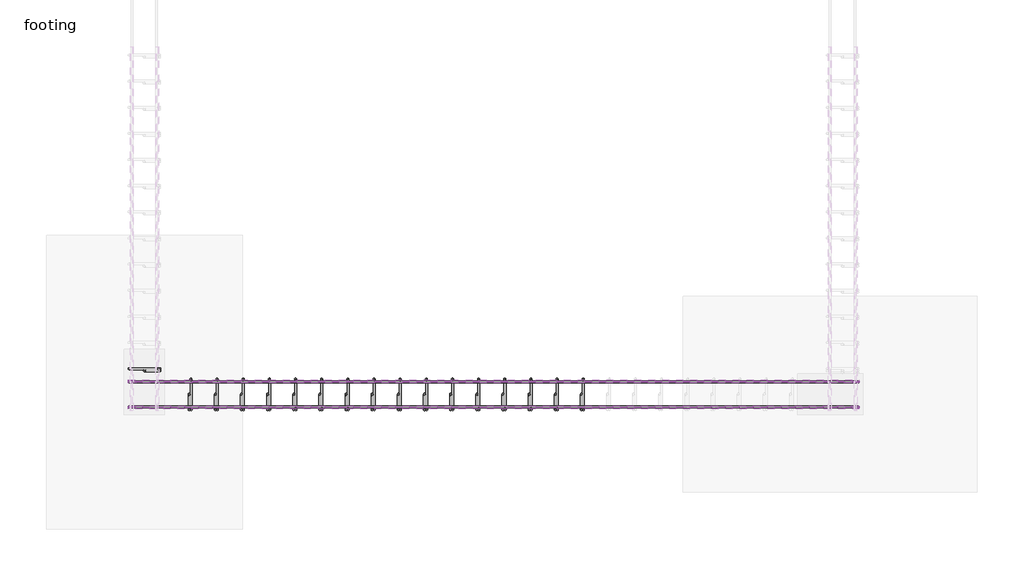
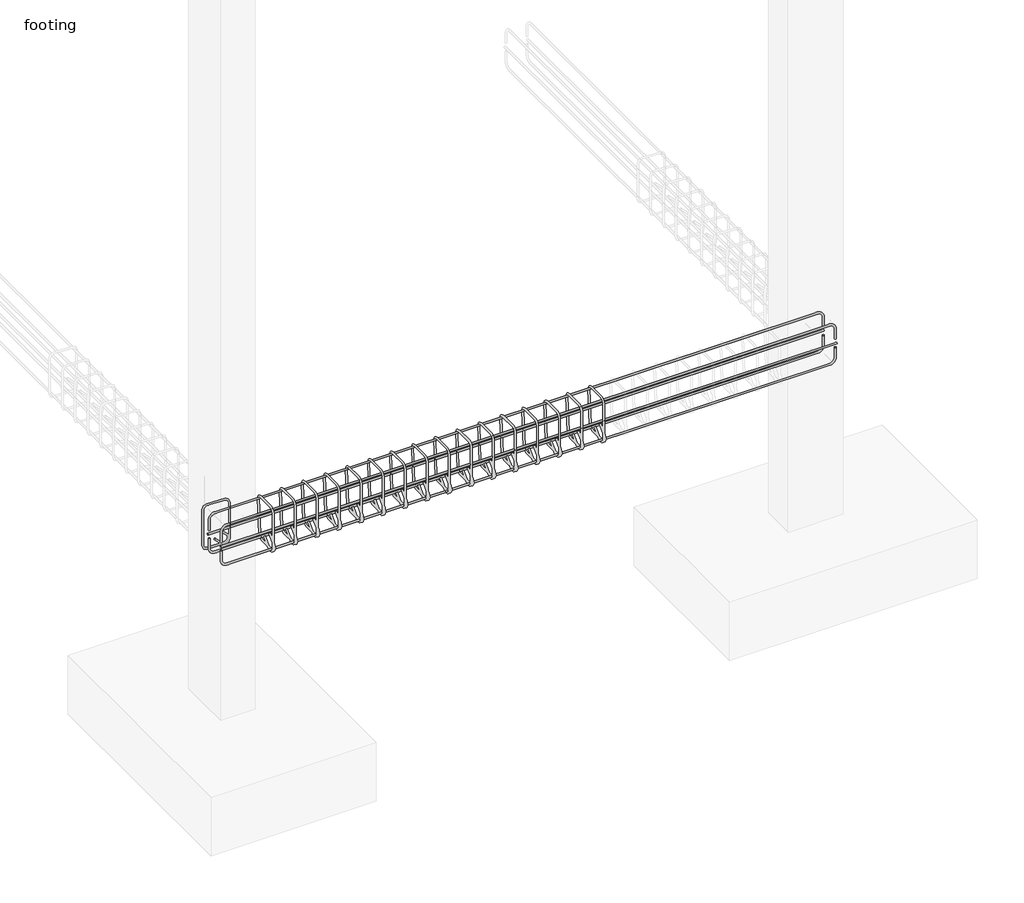
# One storey, part 2 of 21: 23 reinforcing bars.
"""IFC4 building model written with IfcOpenShell, lengths in millimetres."""

from ifc_helpers import new_model, si_unit, point, frame, origin, place, context, project, spatial, polyline, circle_curve, trimmed, segment, composite_curve, element, save
from ifc_brep_helpers import swept_disk

model = new_model("IFC4")

# Units and contexts
model_context = context("Model", 3, world=origin())
ifc_project = project(units=[si_unit("LENGTHUNIT", "METRE", prefix="MILLI")], contexts=[model_context])

# Site, building, storey
site = spatial("IfcSite", under=ifc_project)
building = spatial("IfcBuilding", under=site)
storey = spatial("IfcBuildingStorey", under=building, Name="footing", Elevation=-1524.0)

# Reinforcing bars
placement = place(None, origin())
element("IfcReinforcingBar", 1, at=placement, inside=storey, context=model_context, shape_type="SolidModel", body=[
    swept_disk(composite_curve([segment(polyline([(-11932.2883428, -282.6612868, -310.8825168), (-11932.2883428, -337.5262853, -365.7475153)]), True, "CONTINUOUS"), segment(trimmed(circle_curve(frame((-11932.2883428, -359.9769256, -343.296875), z_axis=(-1.0, 0.0, 0.0), x_axis=(0.0, 22.450640300000032, -22.450640299999975)), 31.75), [point((-11932.2883428, -337.5262853, -365.7475153))], [point((-11932.2883428, -391.7269256, -343.296875))], True, "CARTESIAN"), True, "CONTINUOUS"), segment(polyline([(-11932.2883428, -391.7269256, -343.296875), (-11932.2883428, -391.7269256, -63.103125)]), True, "CONTINUOUS"), segment(trimmed(circle_curve(frame((-11932.2883428, -359.9769256, -63.103125), z_axis=(-1.0, 0.0, 0.0), x_axis=(0.0, -31.75, 0.0)), 31.75), [point((-11932.2883428, -391.7269256, -63.103125))], [point((-11932.2883428, -359.9769256, -31.353125))], True, "CARTESIAN"), True, "CONTINUOUS"), segment(polyline([(-11932.2883428, -359.9769256, -31.353125), (-11932.2883428, -232.1831756, -31.353125)]), True, "CONTINUOUS"), segment(trimmed(circle_curve(frame((-11931.1159328, -232.1831756, -63.0814712), z_axis=(-0.9993179916193466, 0.0, -0.03692629992126919), x_axis=(-1.1724100000010367, 0.0, 31.728346200000004)), 31.75), [point((-11932.2883428, -232.1831756, -31.353125))], [point((-11931.1159328, -200.4331756, -63.0814712))], True, "CARTESIAN"), True, "CONTINUOUS"), segment(polyline([(-11931.1159328, -200.4331756, -63.0814712), (-11920.7607528, -200.4331756, -343.3185288)]), True, "CONTINUOUS"), segment(trimmed(circle_curve(frame((-11920.7607528, -232.1831756, -343.3185288), z_axis=(-0.9993179916193466, 0.0, -0.03692629992126919), x_axis=(0.0, 31.75, 0.0)), 31.75), [point((-11920.7607528, -200.4331756, -343.3185288))], [point((-11919.5883428, -232.1831756, -375.046875))], True, "CARTESIAN"), True, "CONTINUOUS"), segment(polyline([(-11919.5883428, -232.1831756, -375.046875), (-11919.5883428, -359.9769256, -375.046875)]), True, "CONTINUOUS"), segment(trimmed(circle_curve(frame((-11919.5883428, -359.9769256, -343.296875), z_axis=(-1.0, 0.0, 0.0), x_axis=(0.0, 0.0, -31.75)), 31.75), [point((-11919.5883428, -359.9769256, -375.046875))], [point((-11919.5883428, -382.4275659, -320.8462347))], True, "CARTESIAN"), True, "CONTINUOUS"), segment(polyline([(-11919.5883428, -382.4275659, -320.8462347), (-11919.5883428, -327.5625674, -265.9812362)]), True, "CONTINUOUS")], self_intersect=False), 6.35),
])
element("IfcReinforcingBar", 2, at=placement, inside=storey, context=model_context, shape_type="SolidModel", body=[
    swept_disk(composite_curve([segment(polyline([(-11769.5883428, -282.6612868, -310.8825168), (-11769.5883428, -337.5262853, -365.7475153)]), True, "CONTINUOUS"), segment(trimmed(circle_curve(frame((-11769.5883428, -359.9769256, -343.296875), z_axis=(-1.0, 0.0, 0.0), x_axis=(0.0, 22.450640300000032, -22.450640299999975)), 31.75), [point((-11769.5883428, -337.5262853, -365.7475153))], [point((-11769.5883428, -391.7269256, -343.296875))], True, "CARTESIAN"), True, "CONTINUOUS"), segment(polyline([(-11769.5883428, -391.7269256, -343.296875), (-11769.5883428, -391.7269256, -63.103125)]), True, "CONTINUOUS"), segment(trimmed(circle_curve(frame((-11769.5883428, -359.9769256, -63.103125), z_axis=(-1.0, 0.0, 0.0), x_axis=(0.0, -31.75, 0.0)), 31.75), [point((-11769.5883428, -391.7269256, -63.103125))], [point((-11769.5883428, -359.9769256, -31.353125))], True, "CARTESIAN"), True, "CONTINUOUS"), segment(polyline([(-11769.5883428, -359.9769256, -31.353125), (-11769.5883428, -232.1831756, -31.353125)]), True, "CONTINUOUS"), segment(trimmed(circle_curve(frame((-11768.4159328, -232.1831756, -63.0814712), z_axis=(-0.9993179916193466, 0.0, -0.03692629992126919), x_axis=(-1.1724099999992177, 0.0, 31.728346200000004)), 31.75), [point((-11769.5883428, -232.1831756, -31.353125))], [point((-11768.4159328, -200.4331756, -63.0814712))], True, "CARTESIAN"), True, "CONTINUOUS"), segment(polyline([(-11768.4159328, -200.4331756, -63.0814712), (-11758.0607528, -200.4331756, -343.3185288)]), True, "CONTINUOUS"), segment(trimmed(circle_curve(frame((-11758.0607528, -232.1831756, -343.3185288), z_axis=(-0.9993179916193466, 0.0, -0.03692629992126919), x_axis=(0.0, 31.75, 0.0)), 31.75), [point((-11758.0607528, -200.4331756, -343.3185288))], [point((-11756.8883428, -232.1831756, -375.046875))], True, "CARTESIAN"), True, "CONTINUOUS"), segment(polyline([(-11756.8883428, -232.1831756, -375.046875), (-11756.8883428, -359.9769256, -375.046875)]), True, "CONTINUOUS"), segment(trimmed(circle_curve(frame((-11756.8883428, -359.9769256, -343.296875), z_axis=(-1.0, 0.0, 0.0), x_axis=(0.0, 0.0, -31.75)), 31.75), [point((-11756.8883428, -359.9769256, -375.046875))], [point((-11756.8883428, -382.4275659, -320.8462347))], True, "CARTESIAN"), True, "CONTINUOUS"), segment(polyline([(-11756.8883428, -382.4275659, -320.8462347), (-11756.8883428, -327.5625674, -265.9812362)]), True, "CONTINUOUS")], self_intersect=False), 6.35),
])
element("IfcReinforcingBar", 3, at=placement, inside=storey, context=model_context, shape_type="SolidModel", body=[
    swept_disk(composite_curve([segment(polyline([(-11606.8883428, -282.6612868, -310.8825168), (-11606.8883428, -337.5262853, -365.7475153)]), True, "CONTINUOUS"), segment(trimmed(circle_curve(frame((-11606.8883428, -359.9769256, -343.296875), z_axis=(-1.0, 0.0, 0.0), x_axis=(0.0, 22.450640300000032, -22.450640299999975)), 31.75), [point((-11606.8883428, -337.5262853, -365.7475153))], [point((-11606.8883428, -391.7269256, -343.296875))], True, "CARTESIAN"), True, "CONTINUOUS"), segment(polyline([(-11606.8883428, -391.7269256, -343.296875), (-11606.8883428, -391.7269256, -63.103125)]), True, "CONTINUOUS"), segment(trimmed(circle_curve(frame((-11606.8883428, -359.9769256, -63.103125), z_axis=(-1.0, 0.0, 0.0), x_axis=(0.0, -31.75, 0.0)), 31.75), [point((-11606.8883428, -391.7269256, -63.103125))], [point((-11606.8883428, -359.9769256, -31.353125))], True, "CARTESIAN"), True, "CONTINUOUS"), segment(polyline([(-11606.8883428, -359.9769256, -31.353125), (-11606.8883428, -232.1831756, -31.353125)]), True, "CONTINUOUS"), segment(trimmed(circle_curve(frame((-11605.7159328, -232.1831756, -63.0814712), z_axis=(-0.9993179916193466, 0.0, -0.03692629992126919), x_axis=(-1.1724100000010367, 0.0, 31.728346200000004)), 31.75), [point((-11606.8883428, -232.1831756, -31.353125))], [point((-11605.7159328, -200.4331756, -63.0814712))], True, "CARTESIAN"), True, "CONTINUOUS"), segment(polyline([(-11605.7159328, -200.4331756, -63.0814712), (-11595.3607528, -200.4331756, -343.3185288)]), True, "CONTINUOUS"), segment(trimmed(circle_curve(frame((-11595.3607528, -232.1831756, -343.3185288), z_axis=(-0.9993179916193466, 0.0, -0.03692629992126919), x_axis=(0.0, 31.75, 0.0)), 31.75), [point((-11595.3607528, -200.4331756, -343.3185288))], [point((-11594.1883428, -232.1831756, -375.046875))], True, "CARTESIAN"), True, "CONTINUOUS"), segment(polyline([(-11594.1883428, -232.1831756, -375.046875), (-11594.1883428, -359.9769256, -375.046875)]), True, "CONTINUOUS"), segment(trimmed(circle_curve(frame((-11594.1883428, -359.9769256, -343.296875), z_axis=(-1.0, 0.0, 0.0), x_axis=(0.0, 0.0, -31.75)), 31.75), [point((-11594.1883428, -359.9769256, -375.046875))], [point((-11594.1883428, -382.4275659, -320.8462347))], True, "CARTESIAN"), True, "CONTINUOUS"), segment(polyline([(-11594.1883428, -382.4275659, -320.8462347), (-11594.1883428, -327.5625674, -265.9812362)]), True, "CONTINUOUS")], self_intersect=False), 6.35),
])
element("IfcReinforcingBar", 4, at=placement, inside=storey, context=model_context, shape_type="SolidModel", body=[
    swept_disk(composite_curve([segment(polyline([(-11444.1883428, -282.6612868, -310.8825168), (-11444.1883428, -337.5262853, -365.7475153)]), True, "CONTINUOUS"), segment(trimmed(circle_curve(frame((-11444.1883428, -359.9769256, -343.296875), z_axis=(-1.0, 0.0, 0.0), x_axis=(0.0, 22.450640300000032, -22.450640299999975)), 31.75), [point((-11444.1883428, -337.5262853, -365.7475153))], [point((-11444.1883428, -391.7269256, -343.296875))], True, "CARTESIAN"), True, "CONTINUOUS"), segment(polyline([(-11444.1883428, -391.7269256, -343.296875), (-11444.1883428, -391.7269256, -63.103125)]), True, "CONTINUOUS"), segment(trimmed(circle_curve(frame((-11444.1883428, -359.9769256, -63.103125), z_axis=(-1.0, 0.0, 0.0), x_axis=(0.0, -31.75, 0.0)), 31.75), [point((-11444.1883428, -391.7269256, -63.103125))], [point((-11444.1883428, -359.9769256, -31.353125))], True, "CARTESIAN"), True, "CONTINUOUS"), segment(polyline([(-11444.1883428, -359.9769256, -31.353125), (-11444.1883428, -232.1831756, -31.353125)]), True, "CONTINUOUS"), segment(trimmed(circle_curve(frame((-11443.0159328, -232.1831756, -63.0814712), z_axis=(-0.9993179916193466, 0.0, -0.03692629992126919), x_axis=(-1.1724099999992177, 0.0, 31.728346200000004)), 31.75), [point((-11444.1883428, -232.1831756, -31.353125))], [point((-11443.0159328, -200.4331756, -63.0814712))], True, "CARTESIAN"), True, "CONTINUOUS"), segment(polyline([(-11443.0159328, -200.4331756, -63.0814712), (-11432.6607528, -200.4331756, -343.3185288)]), True, "CONTINUOUS"), segment(trimmed(circle_curve(frame((-11432.6607528, -232.1831756, -343.3185288), z_axis=(-0.9993179916193466, 0.0, -0.03692629992126919), x_axis=(0.0, 31.75, 0.0)), 31.75), [point((-11432.6607528, -200.4331756, -343.3185288))], [point((-11431.4883428, -232.1831756, -375.046875))], True, "CARTESIAN"), True, "CONTINUOUS"), segment(polyline([(-11431.4883428, -232.1831756, -375.046875), (-11431.4883428, -359.9769256, -375.046875)]), True, "CONTINUOUS"), segment(trimmed(circle_curve(frame((-11431.4883428, -359.9769256, -343.296875), z_axis=(-1.0, 0.0, 0.0), x_axis=(0.0, 0.0, -31.75)), 31.75), [point((-11431.4883428, -359.9769256, -375.046875))], [point((-11431.4883428, -382.4275659, -320.8462347))], True, "CARTESIAN"), True, "CONTINUOUS"), segment(polyline([(-11431.4883428, -382.4275659, -320.8462347), (-11431.4883428, -327.5625674, -265.9812362)]), True, "CONTINUOUS")], self_intersect=False), 6.35),
])
element("IfcReinforcingBar", 5, at=placement, inside=storey, context=model_context, shape_type="SolidModel", body=[
    swept_disk(composite_curve([segment(polyline([(-11281.4883428, -282.6612868, -310.8825168), (-11281.4883428, -337.5262853, -365.7475153)]), True, "CONTINUOUS"), segment(trimmed(circle_curve(frame((-11281.4883428, -359.9769256, -343.296875), z_axis=(-1.0, 0.0, 0.0), x_axis=(0.0, 22.450640300000032, -22.450640299999975)), 31.75), [point((-11281.4883428, -337.5262853, -365.7475153))], [point((-11281.4883428, -391.7269256, -343.296875))], True, "CARTESIAN"), True, "CONTINUOUS"), segment(polyline([(-11281.4883428, -391.7269256, -343.296875), (-11281.4883428, -391.7269256, -63.103125)]), True, "CONTINUOUS"), segment(trimmed(circle_curve(frame((-11281.4883428, -359.9769256, -63.103125), z_axis=(-1.0, 0.0, 0.0), x_axis=(0.0, -31.75, 0.0)), 31.75), [point((-11281.4883428, -391.7269256, -63.103125))], [point((-11281.4883428, -359.9769256, -31.353125))], True, "CARTESIAN"), True, "CONTINUOUS"), segment(polyline([(-11281.4883428, -359.9769256, -31.353125), (-11281.4883428, -232.1831756, -31.353125)]), True, "CONTINUOUS"), segment(trimmed(circle_curve(frame((-11280.3159328, -232.1831756, -63.0814712), z_axis=(-0.9993179916193466, 0.0, -0.03692629992126919), x_axis=(-1.1724099999992177, 0.0, 31.728346200000004)), 31.75), [point((-11281.4883428, -232.1831756, -31.353125))], [point((-11280.3159328, -200.4331756, -63.0814712))], True, "CARTESIAN"), True, "CONTINUOUS"), segment(polyline([(-11280.3159328, -200.4331756, -63.0814712), (-11269.9607528, -200.4331756, -343.3185288)]), True, "CONTINUOUS"), segment(trimmed(circle_curve(frame((-11269.9607528, -232.1831756, -343.3185288), z_axis=(-0.9993179916193466, 0.0, -0.03692629992126919), x_axis=(0.0, 31.75, 0.0)), 31.75), [point((-11269.9607528, -200.4331756, -343.3185288))], [point((-11268.7883428, -232.1831756, -375.046875))], True, "CARTESIAN"), True, "CONTINUOUS"), segment(polyline([(-11268.7883428, -232.1831756, -375.046875), (-11268.7883428, -359.9769256, -375.046875)]), True, "CONTINUOUS"), segment(trimmed(circle_curve(frame((-11268.7883428, -359.9769256, -343.296875), z_axis=(-1.0, 0.0, 0.0), x_axis=(0.0, 0.0, -31.75)), 31.75), [point((-11268.7883428, -359.9769256, -375.046875))], [point((-11268.7883428, -382.4275659, -320.8462347))], True, "CARTESIAN"), True, "CONTINUOUS"), segment(polyline([(-11268.7883428, -382.4275659, -320.8462347), (-11268.7883428, -327.5625674, -265.9812362)]), True, "CONTINUOUS")], self_intersect=False), 6.35),
])
element("IfcReinforcingBar", 6, at=placement, inside=storey, context=model_context, shape_type="SolidModel", body=[
    swept_disk(composite_curve([segment(polyline([(-11118.7883428, -282.6612868, -310.8825168), (-11118.7883428, -337.5262853, -365.7475153)]), True, "CONTINUOUS"), segment(trimmed(circle_curve(frame((-11118.7883428, -359.9769256, -343.296875), z_axis=(-1.0, 0.0, 0.0), x_axis=(0.0, 22.450640300000032, -22.450640299999975)), 31.75), [point((-11118.7883428, -337.5262853, -365.7475153))], [point((-11118.7883428, -391.7269256, -343.296875))], True, "CARTESIAN"), True, "CONTINUOUS"), segment(polyline([(-11118.7883428, -391.7269256, -343.296875), (-11118.7883428, -391.7269256, -63.103125)]), True, "CONTINUOUS"), segment(trimmed(circle_curve(frame((-11118.7883428, -359.9769256, -63.103125), z_axis=(-1.0, 0.0, 0.0), x_axis=(0.0, -31.75, 0.0)), 31.75), [point((-11118.7883428, -391.7269256, -63.103125))], [point((-11118.7883428, -359.9769256, -31.353125))], True, "CARTESIAN"), True, "CONTINUOUS"), segment(polyline([(-11118.7883428, -359.9769256, -31.353125), (-11118.7883428, -232.1831756, -31.353125)]), True, "CONTINUOUS"), segment(trimmed(circle_curve(frame((-11117.6159328, -232.1831756, -63.0814712), z_axis=(-0.9993179916193466, 0.0, -0.03692629992126919), x_axis=(-1.1724100000010367, 0.0, 31.728346200000004)), 31.75), [point((-11118.7883428, -232.1831756, -31.353125))], [point((-11117.6159328, -200.4331756, -63.0814712))], True, "CARTESIAN"), True, "CONTINUOUS"), segment(polyline([(-11117.6159328, -200.4331756, -63.0814712), (-11107.2607528, -200.4331756, -343.3185288)]), True, "CONTINUOUS"), segment(trimmed(circle_curve(frame((-11107.2607528, -232.1831756, -343.3185288), z_axis=(-0.9993179916193466, 0.0, -0.03692629992126919), x_axis=(0.0, 31.75, 0.0)), 31.75), [point((-11107.2607528, -200.4331756, -343.3185288))], [point((-11106.0883428, -232.1831756, -375.046875))], True, "CARTESIAN"), True, "CONTINUOUS"), segment(polyline([(-11106.0883428, -232.1831756, -375.046875), (-11106.0883428, -359.9769256, -375.046875)]), True, "CONTINUOUS"), segment(trimmed(circle_curve(frame((-11106.0883428, -359.9769256, -343.296875), z_axis=(-1.0, 0.0, 0.0), x_axis=(0.0, 0.0, -31.75)), 31.75), [point((-11106.0883428, -359.9769256, -375.046875))], [point((-11106.0883428, -382.4275659, -320.8462347))], True, "CARTESIAN"), True, "CONTINUOUS"), segment(polyline([(-11106.0883428, -382.4275659, -320.8462347), (-11106.0883428, -327.5625674, -265.9812362)]), True, "CONTINUOUS")], self_intersect=False), 6.35),
])
element("IfcReinforcingBar", 7, at=placement, inside=storey, context=model_context, shape_type="SolidModel", body=[
    swept_disk(composite_curve([segment(polyline([(-10956.0883428, -282.6612868, -310.8825168), (-10956.0883428, -337.5262853, -365.7475153)]), True, "CONTINUOUS"), segment(trimmed(circle_curve(frame((-10956.0883428, -359.9769256, -343.296875), z_axis=(-1.0, 0.0, 0.0), x_axis=(0.0, 22.450640300000032, -22.450640299999975)), 31.75), [point((-10956.0883428, -337.5262853, -365.7475153))], [point((-10956.0883428, -391.7269256, -343.296875))], True, "CARTESIAN"), True, "CONTINUOUS"), segment(polyline([(-10956.0883428, -391.7269256, -343.296875), (-10956.0883428, -391.7269256, -63.103125)]), True, "CONTINUOUS"), segment(trimmed(circle_curve(frame((-10956.0883428, -359.9769256, -63.103125), z_axis=(-1.0, 0.0, 0.0), x_axis=(0.0, -31.75, 0.0)), 31.75), [point((-10956.0883428, -391.7269256, -63.103125))], [point((-10956.0883428, -359.9769256, -31.353125))], True, "CARTESIAN"), True, "CONTINUOUS"), segment(polyline([(-10956.0883428, -359.9769256, -31.353125), (-10956.0883428, -232.1831756, -31.353125)]), True, "CONTINUOUS"), segment(trimmed(circle_curve(frame((-10954.9159328, -232.1831756, -63.0814712), z_axis=(-0.9993179916193466, 0.0, -0.03692629992126919), x_axis=(-1.1724099999992177, 0.0, 31.728346200000004)), 31.75), [point((-10956.0883428, -232.1831756, -31.353125))], [point((-10954.9159328, -200.4331756, -63.0814712))], True, "CARTESIAN"), True, "CONTINUOUS"), segment(polyline([(-10954.9159328, -200.4331756, -63.0814712), (-10944.5607528, -200.4331756, -343.3185288)]), True, "CONTINUOUS"), segment(trimmed(circle_curve(frame((-10944.5607528, -232.1831756, -343.3185288), z_axis=(-0.9993179916193466, 0.0, -0.03692629992126919), x_axis=(0.0, 31.75, 0.0)), 31.75), [point((-10944.5607528, -200.4331756, -343.3185288))], [point((-10943.3883428, -232.1831756, -375.046875))], True, "CARTESIAN"), True, "CONTINUOUS"), segment(polyline([(-10943.3883428, -232.1831756, -375.046875), (-10943.3883428, -359.9769256, -375.046875)]), True, "CONTINUOUS"), segment(trimmed(circle_curve(frame((-10943.3883428, -359.9769256, -343.296875), z_axis=(-1.0, 0.0, 0.0), x_axis=(0.0, 0.0, -31.75)), 31.75), [point((-10943.3883428, -359.9769256, -375.046875))], [point((-10943.3883428, -382.4275659, -320.8462347))], True, "CARTESIAN"), True, "CONTINUOUS"), segment(polyline([(-10943.3883428, -382.4275659, -320.8462347), (-10943.3883428, -327.5625674, -265.9812362)]), True, "CONTINUOUS")], self_intersect=False), 6.35),
])
element("IfcReinforcingBar", 8, at=placement, inside=storey, context=model_context, shape_type="SolidModel", body=[
    swept_disk(composite_curve([segment(polyline([(-10793.3883428, -282.6612868, -310.8825168), (-10793.3883428, -337.5262853, -365.7475153)]), True, "CONTINUOUS"), segment(trimmed(circle_curve(frame((-10793.3883428, -359.9769256, -343.296875), z_axis=(-1.0, 0.0, 0.0), x_axis=(0.0, 22.450640300000032, -22.450640299999975)), 31.75), [point((-10793.3883428, -337.5262853, -365.7475153))], [point((-10793.3883428, -391.7269256, -343.296875))], True, "CARTESIAN"), True, "CONTINUOUS"), segment(polyline([(-10793.3883428, -391.7269256, -343.296875), (-10793.3883428, -391.7269256, -63.103125)]), True, "CONTINUOUS"), segment(trimmed(circle_curve(frame((-10793.3883428, -359.9769256, -63.103125), z_axis=(-1.0, 0.0, 0.0), x_axis=(0.0, -31.75, 0.0)), 31.75), [point((-10793.3883428, -391.7269256, -63.103125))], [point((-10793.3883428, -359.9769256, -31.353125))], True, "CARTESIAN"), True, "CONTINUOUS"), segment(polyline([(-10793.3883428, -359.9769256, -31.353125), (-10793.3883428, -232.1831756, -31.353125)]), True, "CONTINUOUS"), segment(trimmed(circle_curve(frame((-10792.2159328, -232.1831756, -63.0814712), z_axis=(-0.9993179916193466, 0.0, -0.03692629992126919), x_axis=(-1.1724100000010367, 0.0, 31.728346200000004)), 31.75), [point((-10793.3883428, -232.1831756, -31.353125))], [point((-10792.2159328, -200.4331756, -63.0814712))], True, "CARTESIAN"), True, "CONTINUOUS"), segment(polyline([(-10792.2159328, -200.4331756, -63.0814712), (-10781.8607528, -200.4331756, -343.3185288)]), True, "CONTINUOUS"), segment(trimmed(circle_curve(frame((-10781.8607528, -232.1831756, -343.3185288), z_axis=(-0.9993179916193466, 0.0, -0.03692629992126919), x_axis=(0.0, 31.75, 0.0)), 31.75), [point((-10781.8607528, -200.4331756, -343.3185288))], [point((-10780.6883428, -232.1831756, -375.046875))], True, "CARTESIAN"), True, "CONTINUOUS"), segment(polyline([(-10780.6883428, -232.1831756, -375.046875), (-10780.6883428, -359.9769256, -375.046875)]), True, "CONTINUOUS"), segment(trimmed(circle_curve(frame((-10780.6883428, -359.9769256, -343.296875), z_axis=(-1.0, 0.0, 0.0), x_axis=(0.0, 0.0, -31.75)), 31.75), [point((-10780.6883428, -359.9769256, -375.046875))], [point((-10780.6883428, -382.4275659, -320.8462347))], True, "CARTESIAN"), True, "CONTINUOUS"), segment(polyline([(-10780.6883428, -382.4275659, -320.8462347), (-10780.6883428, -327.5625674, -265.9812362)]), True, "CONTINUOUS")], self_intersect=False), 6.35),
])
element("IfcReinforcingBar", 9, at=placement, inside=storey, context=model_context, shape_type="SolidModel", body=[
    swept_disk(composite_curve([segment(polyline([(-10630.6883428, -282.6612868, -310.8825168), (-10630.6883428, -337.5262853, -365.7475153)]), True, "CONTINUOUS"), segment(trimmed(circle_curve(frame((-10630.6883428, -359.9769256, -343.296875), z_axis=(-1.0, 0.0, 0.0), x_axis=(0.0, 22.450640300000032, -22.450640299999975)), 31.75), [point((-10630.6883428, -337.5262853, -365.7475153))], [point((-10630.6883428, -391.7269256, -343.296875))], True, "CARTESIAN"), True, "CONTINUOUS"), segment(polyline([(-10630.6883428, -391.7269256, -343.296875), (-10630.6883428, -391.7269256, -63.103125)]), True, "CONTINUOUS"), segment(trimmed(circle_curve(frame((-10630.6883428, -359.9769256, -63.103125), z_axis=(-1.0, 0.0, 0.0), x_axis=(0.0, -31.75, 0.0)), 31.75), [point((-10630.6883428, -391.7269256, -63.103125))], [point((-10630.6883428, -359.9769256, -31.353125))], True, "CARTESIAN"), True, "CONTINUOUS"), segment(polyline([(-10630.6883428, -359.9769256, -31.353125), (-10630.6883428, -232.1831756, -31.353125)]), True, "CONTINUOUS"), segment(trimmed(circle_curve(frame((-10629.5159328, -232.1831756, -63.0814712), z_axis=(-0.9993179916193466, 0.0, -0.03692629992126919), x_axis=(-1.1724099999992177, 0.0, 31.728346200000004)), 31.75), [point((-10630.6883428, -232.1831756, -31.353125))], [point((-10629.5159328, -200.4331756, -63.0814712))], True, "CARTESIAN"), True, "CONTINUOUS"), segment(polyline([(-10629.5159328, -200.4331756, -63.0814712), (-10619.1607528, -200.4331756, -343.3185288)]), True, "CONTINUOUS"), segment(trimmed(circle_curve(frame((-10619.1607528, -232.1831756, -343.3185288), z_axis=(-0.9993179916193466, 0.0, -0.03692629992126919), x_axis=(0.0, 31.75, 0.0)), 31.75), [point((-10619.1607528, -200.4331756, -343.3185288))], [point((-10617.9883428, -232.1831756, -375.046875))], True, "CARTESIAN"), True, "CONTINUOUS"), segment(polyline([(-10617.9883428, -232.1831756, -375.046875), (-10617.9883428, -359.9769256, -375.046875)]), True, "CONTINUOUS"), segment(trimmed(circle_curve(frame((-10617.9883428, -359.9769256, -343.296875), z_axis=(-1.0, 0.0, 0.0), x_axis=(0.0, 0.0, -31.75)), 31.75), [point((-10617.9883428, -359.9769256, -375.046875))], [point((-10617.9883428, -382.4275659, -320.8462347))], True, "CARTESIAN"), True, "CONTINUOUS"), segment(polyline([(-10617.9883428, -382.4275659, -320.8462347), (-10617.9883428, -327.5625674, -265.9812362)]), True, "CONTINUOUS")], self_intersect=False), 6.35),
])
element("IfcReinforcingBar", 10, at=placement, inside=storey, context=model_context, shape_type="SolidModel", body=[
    swept_disk(composite_curve([segment(polyline([(-10467.9883428, -282.6612868, -310.8825168), (-10467.9883428, -337.5262853, -365.7475153)]), True, "CONTINUOUS"), segment(trimmed(circle_curve(frame((-10467.9883428, -359.9769256, -343.296875), z_axis=(-1.0, 0.0, 0.0), x_axis=(0.0, 22.450640300000032, -22.450640299999975)), 31.75), [point((-10467.9883428, -337.5262853, -365.7475153))], [point((-10467.9883428, -391.7269256, -343.296875))], True, "CARTESIAN"), True, "CONTINUOUS"), segment(polyline([(-10467.9883428, -391.7269256, -343.296875), (-10467.9883428, -391.7269256, -63.103125)]), True, "CONTINUOUS"), segment(trimmed(circle_curve(frame((-10467.9883428, -359.9769256, -63.103125), z_axis=(-1.0, 0.0, 0.0), x_axis=(0.0, -31.75, 0.0)), 31.75), [point((-10467.9883428, -391.7269256, -63.103125))], [point((-10467.9883428, -359.9769256, -31.353125))], True, "CARTESIAN"), True, "CONTINUOUS"), segment(polyline([(-10467.9883428, -359.9769256, -31.353125), (-10467.9883428, -232.1831756, -31.353125)]), True, "CONTINUOUS"), segment(trimmed(circle_curve(frame((-10466.8159328, -232.1831756, -63.0814712), z_axis=(-0.9993179916193466, 0.0, -0.03692629992126919), x_axis=(-1.1724099999992177, 0.0, 31.728346200000004)), 31.75), [point((-10467.9883428, -232.1831756, -31.353125))], [point((-10466.8159328, -200.4331756, -63.0814712))], True, "CARTESIAN"), True, "CONTINUOUS"), segment(polyline([(-10466.8159328, -200.4331756, -63.0814712), (-10456.4607528, -200.4331756, -343.3185288)]), True, "CONTINUOUS"), segment(trimmed(circle_curve(frame((-10456.4607528, -232.1831756, -343.3185288), z_axis=(-0.9993179916193466, 0.0, -0.03692629992126919), x_axis=(0.0, 31.75, 0.0)), 31.75), [point((-10456.4607528, -200.4331756, -343.3185288))], [point((-10455.2883428, -232.1831756, -375.046875))], True, "CARTESIAN"), True, "CONTINUOUS"), segment(polyline([(-10455.2883428, -232.1831756, -375.046875), (-10455.2883428, -359.9769256, -375.046875)]), True, "CONTINUOUS"), segment(trimmed(circle_curve(frame((-10455.2883428, -359.9769256, -343.296875), z_axis=(-1.0, 0.0, 0.0), x_axis=(0.0, 0.0, -31.75)), 31.75), [point((-10455.2883428, -359.9769256, -375.046875))], [point((-10455.2883428, -382.4275659, -320.8462347))], True, "CARTESIAN"), True, "CONTINUOUS"), segment(polyline([(-10455.2883428, -382.4275659, -320.8462347), (-10455.2883428, -327.5625674, -265.9812362)]), True, "CONTINUOUS")], self_intersect=False), 6.35),
])
element("IfcReinforcingBar", 11, at=placement, inside=storey, context=model_context, shape_type="SolidModel", body=[
    swept_disk(composite_curve([segment(polyline([(-10305.2883428, -282.6612868, -310.8825168), (-10305.2883428, -337.5262853, -365.7475153)]), True, "CONTINUOUS"), segment(trimmed(circle_curve(frame((-10305.2883428, -359.9769256, -343.296875), z_axis=(-1.0, 0.0, 0.0), x_axis=(0.0, 22.450640300000032, -22.450640299999975)), 31.75), [point((-10305.2883428, -337.5262853, -365.7475153))], [point((-10305.2883428, -391.7269256, -343.296875))], True, "CARTESIAN"), True, "CONTINUOUS"), segment(polyline([(-10305.2883428, -391.7269256, -343.296875), (-10305.2883428, -391.7269256, -63.103125)]), True, "CONTINUOUS"), segment(trimmed(circle_curve(frame((-10305.2883428, -359.9769256, -63.103125), z_axis=(-1.0, 0.0, 0.0), x_axis=(0.0, -31.75, 0.0)), 31.75), [point((-10305.2883428, -391.7269256, -63.103125))], [point((-10305.2883428, -359.9769256, -31.353125))], True, "CARTESIAN"), True, "CONTINUOUS"), segment(polyline([(-10305.2883428, -359.9769256, -31.353125), (-10305.2883428, -232.1831756, -31.353125)]), True, "CONTINUOUS"), segment(trimmed(circle_curve(frame((-10304.1159328, -232.1831756, -63.0814712), z_axis=(-0.9993179916193466, 0.0, -0.03692629992126919), x_axis=(-1.1724100000010367, 0.0, 31.728346200000004)), 31.75), [point((-10305.2883428, -232.1831756, -31.353125))], [point((-10304.1159328, -200.4331756, -63.0814712))], True, "CARTESIAN"), True, "CONTINUOUS"), segment(polyline([(-10304.1159328, -200.4331756, -63.0814712), (-10293.7607528, -200.4331756, -343.3185288)]), True, "CONTINUOUS"), segment(trimmed(circle_curve(frame((-10293.7607528, -232.1831756, -343.3185288), z_axis=(-0.9993179916193466, 0.0, -0.03692629992126919), x_axis=(0.0, 31.75, 0.0)), 31.75), [point((-10293.7607528, -200.4331756, -343.3185288))], [point((-10292.5883428, -232.1831756, -375.046875))], True, "CARTESIAN"), True, "CONTINUOUS"), segment(polyline([(-10292.5883428, -232.1831756, -375.046875), (-10292.5883428, -359.9769256, -375.046875)]), True, "CONTINUOUS"), segment(trimmed(circle_curve(frame((-10292.5883428, -359.9769256, -343.296875), z_axis=(-1.0, 0.0, 0.0), x_axis=(0.0, 0.0, -31.75)), 31.75), [point((-10292.5883428, -359.9769256, -375.046875))], [point((-10292.5883428, -382.4275659, -320.8462347))], True, "CARTESIAN"), True, "CONTINUOUS"), segment(polyline([(-10292.5883428, -382.4275659, -320.8462347), (-10292.5883428, -327.5625674, -265.9812362)]), True, "CONTINUOUS")], self_intersect=False), 6.35),
])
element("IfcReinforcingBar", 12, at=placement, inside=storey, context=model_context, shape_type="SolidModel", body=[
    swept_disk(composite_curve([segment(polyline([(-10142.5883428, -282.6612868, -310.8825168), (-10142.5883428, -337.5262853, -365.7475153)]), True, "CONTINUOUS"), segment(trimmed(circle_curve(frame((-10142.5883428, -359.9769256, -343.296875), z_axis=(-1.0, 0.0, 0.0), x_axis=(0.0, 22.450640300000032, -22.450640299999975)), 31.75), [point((-10142.5883428, -337.5262853, -365.7475153))], [point((-10142.5883428, -391.7269256, -343.296875))], True, "CARTESIAN"), True, "CONTINUOUS"), segment(polyline([(-10142.5883428, -391.7269256, -343.296875), (-10142.5883428, -391.7269256, -63.103125)]), True, "CONTINUOUS"), segment(trimmed(circle_curve(frame((-10142.5883428, -359.9769256, -63.103125), z_axis=(-1.0, 0.0, 0.0), x_axis=(0.0, -31.75, 0.0)), 31.75), [point((-10142.5883428, -391.7269256, -63.103125))], [point((-10142.5883428, -359.9769256, -31.353125))], True, "CARTESIAN"), True, "CONTINUOUS"), segment(polyline([(-10142.5883428, -359.9769256, -31.353125), (-10142.5883428, -232.1831756, -31.353125)]), True, "CONTINUOUS"), segment(trimmed(circle_curve(frame((-10141.4159328, -232.1831756, -63.0814712), z_axis=(-0.9993179916193466, 0.0, -0.03692629992126919), x_axis=(-1.1724099999992177, 0.0, 31.728346200000004)), 31.75), [point((-10142.5883428, -232.1831756, -31.353125))], [point((-10141.4159328, -200.4331756, -63.0814712))], True, "CARTESIAN"), True, "CONTINUOUS"), segment(polyline([(-10141.4159328, -200.4331756, -63.0814712), (-10131.0607528, -200.4331756, -343.3185288)]), True, "CONTINUOUS"), segment(trimmed(circle_curve(frame((-10131.0607528, -232.1831756, -343.3185288), z_axis=(-0.9993179916193466, 0.0, -0.03692629992126919), x_axis=(0.0, 31.75, 0.0)), 31.75), [point((-10131.0607528, -200.4331756, -343.3185288))], [point((-10129.8883428, -232.1831756, -375.046875))], True, "CARTESIAN"), True, "CONTINUOUS"), segment(polyline([(-10129.8883428, -232.1831756, -375.046875), (-10129.8883428, -359.9769256, -375.046875)]), True, "CONTINUOUS"), segment(trimmed(circle_curve(frame((-10129.8883428, -359.9769256, -343.296875), z_axis=(-1.0, 0.0, 0.0), x_axis=(0.0, 0.0, -31.75)), 31.75), [point((-10129.8883428, -359.9769256, -375.046875))], [point((-10129.8883428, -382.4275659, -320.8462347))], True, "CARTESIAN"), True, "CONTINUOUS"), segment(polyline([(-10129.8883428, -382.4275659, -320.8462347), (-10129.8883428, -327.5625674, -265.9812362)]), True, "CONTINUOUS")], self_intersect=False), 6.35),
])
element("IfcReinforcingBar", 13, at=placement, inside=storey, context=model_context, shape_type="SolidModel", body=[
    swept_disk(composite_curve([segment(polyline([(-9979.8883428, -282.6612868, -310.8825168), (-9979.8883428, -337.5262853, -365.7475153)]), True, "CONTINUOUS"), segment(trimmed(circle_curve(frame((-9979.8883428, -359.9769256, -343.296875), z_axis=(-1.0, 0.0, 0.0), x_axis=(0.0, 22.450640300000032, -22.450640299999975)), 31.75), [point((-9979.8883428, -337.5262853, -365.7475153))], [point((-9979.8883428, -391.7269256, -343.296875))], True, "CARTESIAN"), True, "CONTINUOUS"), segment(polyline([(-9979.8883428, -391.7269256, -343.296875), (-9979.8883428, -391.7269256, -63.103125)]), True, "CONTINUOUS"), segment(trimmed(circle_curve(frame((-9979.8883428, -359.9769256, -63.103125), z_axis=(-1.0, 0.0, 0.0), x_axis=(0.0, -31.75, 0.0)), 31.75), [point((-9979.8883428, -391.7269256, -63.103125))], [point((-9979.8883428, -359.9769256, -31.353125))], True, "CARTESIAN"), True, "CONTINUOUS"), segment(polyline([(-9979.8883428, -359.9769256, -31.353125), (-9979.8883428, -232.1831756, -31.353125)]), True, "CONTINUOUS"), segment(trimmed(circle_curve(frame((-9978.7159328, -232.1831756, -63.0814712), z_axis=(-0.9993179916193466, 0.0, -0.03692629992126919), x_axis=(-1.1724100000010367, 0.0, 31.728346200000004)), 31.75), [point((-9979.8883428, -232.1831756, -31.353125))], [point((-9978.7159328, -200.4331756, -63.0814712))], True, "CARTESIAN"), True, "CONTINUOUS"), segment(polyline([(-9978.7159328, -200.4331756, -63.0814712), (-9968.3607528, -200.4331756, -343.3185288)]), True, "CONTINUOUS"), segment(trimmed(circle_curve(frame((-9968.3607528, -232.1831756, -343.3185288), z_axis=(-0.9993179916193466, 0.0, -0.03692629992126919), x_axis=(0.0, 31.75, 0.0)), 31.75), [point((-9968.3607528, -200.4331756, -343.3185288))], [point((-9967.1883428, -232.1831756, -375.046875))], True, "CARTESIAN"), True, "CONTINUOUS"), segment(polyline([(-9967.1883428, -232.1831756, -375.046875), (-9967.1883428, -359.9769256, -375.046875)]), True, "CONTINUOUS"), segment(trimmed(circle_curve(frame((-9967.1883428, -359.9769256, -343.296875), z_axis=(-1.0, 0.0, 0.0), x_axis=(0.0, 0.0, -31.75)), 31.75), [point((-9967.1883428, -359.9769256, -375.046875))], [point((-9967.1883428, -382.4275659, -320.8462347))], True, "CARTESIAN"), True, "CONTINUOUS"), segment(polyline([(-9967.1883428, -382.4275659, -320.8462347), (-9967.1883428, -327.5625674, -265.9812362)]), True, "CONTINUOUS")], self_intersect=False), 6.35),
])
element("IfcReinforcingBar", 14, at=placement, inside=storey, context=model_context, shape_type="SolidModel", body=[
    swept_disk(composite_curve([segment(polyline([(-9817.1883428, -282.6612868, -310.8825168), (-9817.1883428, -337.5262853, -365.7475153)]), True, "CONTINUOUS"), segment(trimmed(circle_curve(frame((-9817.1883428, -359.9769256, -343.296875), z_axis=(-1.0, 0.0, 0.0), x_axis=(0.0, 22.450640300000032, -22.450640299999975)), 31.75), [point((-9817.1883428, -337.5262853, -365.7475153))], [point((-9817.1883428, -391.7269256, -343.296875))], True, "CARTESIAN"), True, "CONTINUOUS"), segment(polyline([(-9817.1883428, -391.7269256, -343.296875), (-9817.1883428, -391.7269256, -63.103125)]), True, "CONTINUOUS"), segment(trimmed(circle_curve(frame((-9817.1883428, -359.9769256, -63.103125), z_axis=(-1.0, 0.0, 0.0), x_axis=(0.0, -31.75, 0.0)), 31.75), [point((-9817.1883428, -391.7269256, -63.103125))], [point((-9817.1883428, -359.9769256, -31.353125))], True, "CARTESIAN"), True, "CONTINUOUS"), segment(polyline([(-9817.1883428, -359.9769256, -31.353125), (-9817.1883428, -232.1831756, -31.353125)]), True, "CONTINUOUS"), segment(trimmed(circle_curve(frame((-9816.0159328, -232.1831756, -63.0814712), z_axis=(-0.9993179916193466, 0.0, -0.03692629992126919), x_axis=(-1.1724099999992177, 0.0, 31.728346200000004)), 31.75), [point((-9817.1883428, -232.1831756, -31.353125))], [point((-9816.0159328, -200.4331756, -63.0814712))], True, "CARTESIAN"), True, "CONTINUOUS"), segment(polyline([(-9816.0159328, -200.4331756, -63.0814712), (-9805.6607528, -200.4331756, -343.3185288)]), True, "CONTINUOUS"), segment(trimmed(circle_curve(frame((-9805.6607528, -232.1831756, -343.3185288), z_axis=(-0.9993179916193466, 0.0, -0.03692629992126919), x_axis=(0.0, 31.75, 0.0)), 31.75), [point((-9805.6607528, -200.4331756, -343.3185288))], [point((-9804.4883428, -232.1831756, -375.046875))], True, "CARTESIAN"), True, "CONTINUOUS"), segment(polyline([(-9804.4883428, -232.1831756, -375.046875), (-9804.4883428, -359.9769256, -375.046875)]), True, "CONTINUOUS"), segment(trimmed(circle_curve(frame((-9804.4883428, -359.9769256, -343.296875), z_axis=(-1.0, 0.0, 0.0), x_axis=(0.0, 0.0, -31.75)), 31.75), [point((-9804.4883428, -359.9769256, -375.046875))], [point((-9804.4883428, -382.4275659, -320.8462347))], True, "CARTESIAN"), True, "CONTINUOUS"), segment(polyline([(-9804.4883428, -382.4275659, -320.8462347), (-9804.4883428, -327.5625674, -265.9812362)]), True, "CONTINUOUS")], self_intersect=False), 6.35),
])
element("IfcReinforcingBar", 15, at=placement, inside=storey, context=model_context, shape_type="SolidModel", body=[
    swept_disk(composite_curve([segment(polyline([(-9654.4883428, -282.6612868, -310.8825168), (-9654.4883428, -337.5262853, -365.7475153)]), True, "CONTINUOUS"), segment(trimmed(circle_curve(frame((-9654.4883428, -359.9769256, -343.296875), z_axis=(-1.0, 0.0, 0.0), x_axis=(0.0, 22.450640300000032, -22.450640299999975)), 31.75), [point((-9654.4883428, -337.5262853, -365.7475153))], [point((-9654.4883428, -391.7269256, -343.296875))], True, "CARTESIAN"), True, "CONTINUOUS"), segment(polyline([(-9654.4883428, -391.7269256, -343.296875), (-9654.4883428, -391.7269256, -63.103125)]), True, "CONTINUOUS"), segment(trimmed(circle_curve(frame((-9654.4883428, -359.9769256, -63.103125), z_axis=(-1.0, 0.0, 0.0), x_axis=(0.0, -31.75, 0.0)), 31.75), [point((-9654.4883428, -391.7269256, -63.103125))], [point((-9654.4883428, -359.9769256, -31.353125))], True, "CARTESIAN"), True, "CONTINUOUS"), segment(polyline([(-9654.4883428, -359.9769256, -31.353125), (-9654.4883428, -232.1831756, -31.353125)]), True, "CONTINUOUS"), segment(trimmed(circle_curve(frame((-9653.3159328, -232.1831756, -63.0814712), z_axis=(-0.9993179916193466, 0.0, -0.03692629992126919), x_axis=(-1.1724099999992177, 0.0, 31.728346200000004)), 31.75), [point((-9654.4883428, -232.1831756, -31.353125))], [point((-9653.3159328, -200.4331756, -63.0814712))], True, "CARTESIAN"), True, "CONTINUOUS"), segment(polyline([(-9653.3159328, -200.4331756, -63.0814712), (-9642.9607528, -200.4331756, -343.3185288)]), True, "CONTINUOUS"), segment(trimmed(circle_curve(frame((-9642.9607528, -232.1831756, -343.3185288), z_axis=(-0.9993179916193466, 0.0, -0.03692629992126919), x_axis=(0.0, 31.75, 0.0)), 31.75), [point((-9642.9607528, -200.4331756, -343.3185288))], [point((-9641.7883428, -232.1831756, -375.046875))], True, "CARTESIAN"), True, "CONTINUOUS"), segment(polyline([(-9641.7883428, -232.1831756, -375.046875), (-9641.7883428, -359.9769256, -375.046875)]), True, "CONTINUOUS"), segment(trimmed(circle_curve(frame((-9641.7883428, -359.9769256, -343.296875), z_axis=(-1.0, 0.0, 0.0), x_axis=(0.0, 0.0, -31.75)), 31.75), [point((-9641.7883428, -359.9769256, -375.046875))], [point((-9641.7883428, -382.4275659, -320.8462347))], True, "CARTESIAN"), True, "CONTINUOUS"), segment(polyline([(-9641.7883428, -382.4275659, -320.8462347), (-9641.7883428, -327.5625674, -265.9812362)]), True, "CONTINUOUS")], self_intersect=False), 6.35),
])
element("IfcReinforcingBar", 16, at=placement, inside=storey, context=model_context, shape_type="SolidModel", body=[
    swept_disk(composite_curve([segment(polyline([(-9491.7883428, -282.6612868, -310.8825168), (-9491.7883428, -337.5262853, -365.7475153)]), True, "CONTINUOUS"), segment(trimmed(circle_curve(frame((-9491.7883428, -359.9769256, -343.296875), z_axis=(-1.0, 0.0, 0.0), x_axis=(0.0, 22.450640300000032, -22.450640299999975)), 31.75), [point((-9491.7883428, -337.5262853, -365.7475153))], [point((-9491.7883428, -391.7269256, -343.296875))], True, "CARTESIAN"), True, "CONTINUOUS"), segment(polyline([(-9491.7883428, -391.7269256, -343.296875), (-9491.7883428, -391.7269256, -63.103125)]), True, "CONTINUOUS"), segment(trimmed(circle_curve(frame((-9491.7883428, -359.9769256, -63.103125), z_axis=(-1.0, 0.0, 0.0), x_axis=(0.0, -31.75, 0.0)), 31.75), [point((-9491.7883428, -391.7269256, -63.103125))], [point((-9491.7883428, -359.9769256, -31.353125))], True, "CARTESIAN"), True, "CONTINUOUS"), segment(polyline([(-9491.7883428, -359.9769256, -31.353125), (-9491.7883428, -232.1831756, -31.353125)]), True, "CONTINUOUS"), segment(trimmed(circle_curve(frame((-9490.6159328, -232.1831756, -63.0814712), z_axis=(-0.9993179916193466, 0.0, -0.03692629992126919), x_axis=(-1.1724100000010367, 0.0, 31.728346200000004)), 31.75), [point((-9491.7883428, -232.1831756, -31.353125))], [point((-9490.6159328, -200.4331756, -63.0814712))], True, "CARTESIAN"), True, "CONTINUOUS"), segment(polyline([(-9490.6159328, -200.4331756, -63.0814712), (-9480.2607528, -200.4331756, -343.3185288)]), True, "CONTINUOUS"), segment(trimmed(circle_curve(frame((-9480.2607528, -232.1831756, -343.3185288), z_axis=(-0.9993179916193466, 0.0, -0.03692629992126919), x_axis=(0.0, 31.75, 0.0)), 31.75), [point((-9480.2607528, -200.4331756, -343.3185288))], [point((-9479.0883428, -232.1831756, -375.046875))], True, "CARTESIAN"), True, "CONTINUOUS"), segment(polyline([(-9479.0883428, -232.1831756, -375.046875), (-9479.0883428, -359.9769256, -375.046875)]), True, "CONTINUOUS"), segment(trimmed(circle_curve(frame((-9479.0883428, -359.9769256, -343.296875), z_axis=(-1.0, 0.0, 0.0), x_axis=(0.0, 0.0, -31.75)), 31.75), [point((-9479.0883428, -359.9769256, -375.046875))], [point((-9479.0883428, -382.4275659, -320.8462347))], True, "CARTESIAN"), True, "CONTINUOUS"), segment(polyline([(-9479.0883428, -382.4275659, -320.8462347), (-9479.0883428, -327.5625674, -265.9812362)]), True, "CONTINUOUS")], self_intersect=False), 6.35),
])
element("IfcReinforcingBar", 17, at=placement, inside=storey, context=model_context, shape_type="SolidModel", body=[
    swept_disk(composite_curve([segment(polyline([(-7770.5521673, -218.7127914, -170.2827408), (-7770.5521673, -218.7127914, -94.0827408)]), True, "CONTINUOUS"), segment(trimmed(circle_curve(frame((-7815.0021673, -218.7127914, -94.0827408), z_axis=(0.0, -1.0, 0.0), x_axis=(44.44999999999982, 0.0, 0.0)), 44.45), [point((-7770.5521673, -218.7127914, -94.0827408))], [point((-7815.0021673, -218.7127914, -49.6327408))], True, "CARTESIAN"), True, "CONTINUOUS"), segment(polyline([(-7815.0021673, -218.7127914, -49.6327408), (-12260.7959173, -218.7127914, -49.6327408)]), True, "CONTINUOUS"), segment(trimmed(circle_curve(frame((-12260.7959173, -218.7127914, -94.0827408), z_axis=(0.0, -1.0, 0.0), x_axis=(0.0, 0.0, 44.449999999999996)), 44.45), [point((-12260.7959173, -218.7127914, -49.6327408))], [point((-12305.2459173, -218.7127914, -94.0827408))], True, "CARTESIAN"), True, "CONTINUOUS"), segment(polyline([(-12305.2459173, -218.7127914, -94.0827408), (-12305.2459173, -218.7127914, -170.2827408)]), True, "CONTINUOUS")], self_intersect=False), 6.35),
])
element("IfcReinforcingBar", 18, at=placement, inside=storey, context=model_context, shape_type="SolidModel", body=[
    swept_disk(composite_curve([segment(polyline([(-7770.5521673, -373.4473098, -170.2827408), (-7770.5521673, -373.4473098, -94.0827408)]), True, "CONTINUOUS"), segment(trimmed(circle_curve(frame((-7815.0021673, -373.4473098, -94.0827408), z_axis=(0.0, -1.0, 2.038997073047455e-12), x_axis=(44.44999999999982, 0.0, 0.0)), 44.45), [point((-7770.5521673, -373.4473098, -94.0827408))], [point((-7815.0021673, -373.4473098, -49.6327408))], True, "CARTESIAN"), True, "CONTINUOUS"), segment(polyline([(-7815.0021673, -373.4473098, -49.6327408), (-12260.7959173, -373.4473098, -49.6327408)]), True, "CONTINUOUS"), segment(trimmed(circle_curve(frame((-12260.7959173, -373.4473098, -94.0827408), z_axis=(0.0, -1.0, 2.038997073047455e-12), x_axis=(0.0, 0.0, 44.449999999999996)), 44.45), [point((-12260.7959173, -373.4473098, -49.6327408))], [point((-12305.2459173, -373.4473098, -94.0827408))], True, "CARTESIAN"), True, "CONTINUOUS"), segment(polyline([(-12305.2459173, -373.4473098, -94.0827408), (-12305.2459173, -373.4473098, -170.2827408)]), True, "CONTINUOUS")], self_intersect=False), 6.35),
])
element("IfcReinforcingBar", 19, at=placement, inside=storey, context=model_context, shape_type="SolidModel", body=[
    swept_disk(composite_curve([segment(polyline([(-7770.5521673, -218.7127914, -236.1172592), (-7770.5521673, -218.7127914, -312.3172592)]), True, "CONTINUOUS"), segment(trimmed(circle_curve(frame((-7815.0021673, -218.7127914, -312.3172592), z_axis=(0.0, 1.0, 0.0), x_axis=(44.44999999999982, 0.0, 0.0)), 44.45), [point((-7770.5521673, -218.7127914, -312.3172592))], [point((-7815.0021673, -218.7127914, -356.7672592))], True, "CARTESIAN"), True, "CONTINUOUS"), segment(polyline([(-7815.0021673, -218.7127914, -356.7672592), (-12260.7959173, -218.7127914, -356.7672592)]), True, "CONTINUOUS"), segment(trimmed(circle_curve(frame((-12260.7959173, -218.7127914, -312.3172592), z_axis=(0.0, 1.0, 0.0), x_axis=(0.0, 0.0, -44.44999999999999)), 44.45), [point((-12260.7959173, -218.7127914, -356.7672592))], [point((-12305.2459173, -218.7127914, -312.3172592))], True, "CARTESIAN"), True, "CONTINUOUS"), segment(polyline([(-12305.2459173, -218.7127914, -312.3172592), (-12305.2459173, -218.7127914, -236.1172592)]), True, "CONTINUOUS")], self_intersect=False), 6.35),
])
element("IfcReinforcingBar", 20, at=placement, inside=storey, context=model_context, shape_type="SolidModel", body=[
    swept_disk(composite_curve([segment(polyline([(-7770.5521673, -373.4473098, -236.1172592), (-7770.5521673, -373.4473098, -312.3172592)]), True, "CONTINUOUS"), segment(trimmed(circle_curve(frame((-7815.0021673, -373.4473098, -312.3172592), z_axis=(0.0, 1.0, 2.1166279873208456e-12), x_axis=(44.44999999999982, 0.0, 0.0)), 44.45), [point((-7770.5521673, -373.4473098, -312.3172592))], [point((-7815.0021673, -373.4473098, -356.7672592))], True, "CARTESIAN"), True, "CONTINUOUS"), segment(polyline([(-7815.0021673, -373.4473098, -356.7672592), (-12260.7959173, -373.4473098, -356.7672592)]), True, "CONTINUOUS"), segment(trimmed(circle_curve(frame((-12260.7959173, -373.4473098, -312.3172592), z_axis=(0.0, 1.0, 2.1166279873208456e-12), x_axis=(0.0, 0.0, -44.44999999999999)), 44.45), [point((-12260.7959173, -373.4473098, -356.7672592))], [point((-12305.2459173, -373.4473098, -312.3172592))], True, "CARTESIAN"), True, "CONTINUOUS"), segment(polyline([(-12305.2459173, -373.4473098, -312.3172592), (-12305.2459173, -373.4473098, -236.1172592)]), True, "CONTINUOUS")], self_intersect=False), 6.35),
])
element("IfcReinforcingBar", 21, at=placement, inside=storey, context=model_context, shape_type="SolidModel", body=[
    swept_disk(composite_curve([segment(polyline([(-7764.2021673, -213.1331756, -203.2), (-12311.5959173, -213.1331756, -203.2)]), True, "CONTINUOUS")], self_intersect=False), 6.35),
])
element("IfcReinforcingBar", 22, at=placement, inside=storey, context=model_context, shape_type="SolidModel", body=[
    swept_disk(composite_curve([segment(polyline([(-7764.2021673, -379.0269256, -203.2), (-12311.5959173, -379.0269256, -203.2)]), True, "CONTINUOUS")], self_intersect=False), 6.35),
])
element("IfcReinforcingBar", 23, at=placement, inside=storey, context=model_context, shape_type="SolidModel", body=[
    swept_disk(composite_curve([segment(polyline([(-12178.1165254, -135.8043927, -265.9812362), (-12123.251527, -135.8043927, -320.8462347)]), True, "CONTINUOUS"), segment(trimmed(circle_curve(frame((-12145.7021673, -135.8043927, -343.296875), z_axis=(0.0, 1.0, 0.0), x_axis=(22.450640299999577, 0.0, 22.450640299999975)), 31.75), [point((-12123.251527, -135.8043927, -320.8462347))], [point((-12145.7021673, -135.8043927, -375.046875))], True, "CARTESIAN"), True, "CONTINUOUS"), segment(polyline([(-12145.7021673, -135.8043927, -375.046875), (-12273.4959173, -135.8043927, -375.046875)]), True, "CONTINUOUS"), segment(trimmed(circle_curve(frame((-12273.4959173, -135.8043927, -343.296875), z_axis=(0.0, 1.0, 0.0), x_axis=(0.0, 0.0, -31.75)), 31.75), [point((-12273.4959173, -135.8043927, -375.046875))], [point((-12305.2459173, -135.8043927, -343.296875))], True, "CARTESIAN"), True, "CONTINUOUS"), segment(polyline([(-12305.2459173, -135.8043927, -343.296875), (-12305.2459173, -135.8043927, -63.103125)]), True, "CONTINUOUS"), segment(trimmed(circle_curve(frame((-12273.565658, -137.9076464, -63.103125), z_axis=(0.0662442117686417, 0.9978034397651431, 0.0), x_axis=(-31.680259300001126, 2.1032537000000104, 0.0)), 31.75), [point((-12305.2459173, -135.8043927, -63.103125))], [point((-12273.565658, -137.9076464, -31.353125))], True, "CARTESIAN"), True, "CONTINUOUS"), segment(polyline([(-12273.565658, -137.9076464, -31.353125), (-12145.6324265, -146.401139, -31.353125)]), True, "CONTINUOUS"), segment(trimmed(circle_curve(frame((-12145.6324265, -146.401139, -63.103125), z_axis=(0.06624421176864169, 0.997803439765143, 0.0), x_axis=(0.0, 0.0, 31.75)), 31.75), [point((-12145.6324265, -146.401139, -31.353125))], [point((-12113.9521673, -148.5043927, -63.103125))], True, "CARTESIAN"), True, "CONTINUOUS"), segment(polyline([(-12113.9521673, -148.5043927, -63.103125), (-12113.9521673, -148.5043927, -343.296875)]), True, "CONTINUOUS"), segment(trimmed(circle_curve(frame((-12145.7021673, -148.5043927, -343.296875), z_axis=(0.0, 1.0, 0.0), x_axis=(31.75, 0.0, 0.0)), 31.75), [point((-12113.9521673, -148.5043927, -343.296875))], [point((-12168.1528076, -148.5043927, -365.7475153))], True, "CARTESIAN"), True, "CONTINUOUS"), segment(polyline([(-12168.1528076, -148.5043927, -365.7475153), (-12223.017806, -148.5043927, -310.8825168)]), True, "CONTINUOUS")], self_intersect=False), 6.35),
])

save(model, "model.ifc")

# Revit data of these elements
# Elements 1, 2, 3, 4, 5, 6, 7, 8, 9, 10, 11, 12, 13, 14, 15, 16, 17, 18, 19, 20, 21, 22, 23 (IfcReinforcingBar)
#   Phase Created = New Construction
